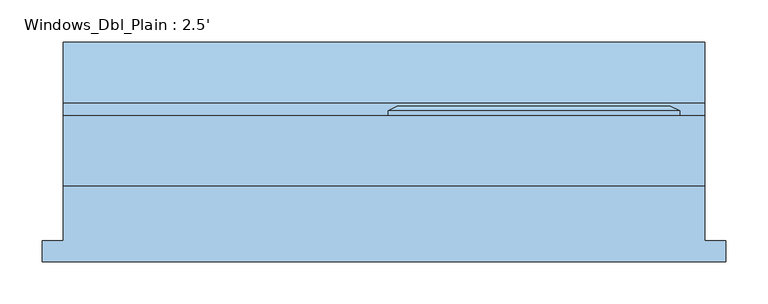
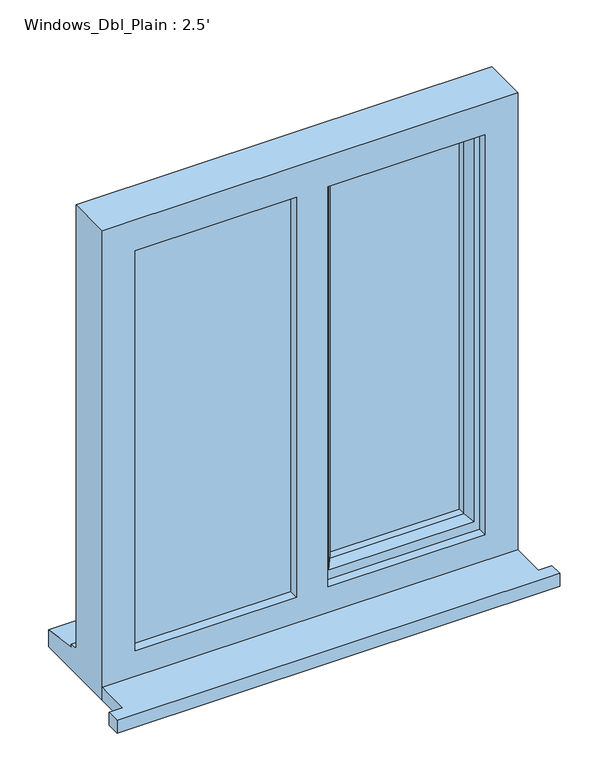
"""IFC4 building model written with IfcOpenShell, lengths in millimetres: window geometry, Windows_Dbl_Plain : 2.5'."""

from ifc_helpers import new_model, si_unit, frame, origin, place, context, project, spatial, polyline, outline, extrude, faceted_brep, source, transform, mapped, element, save


def windows_dbl_plain_2_5_52f1e8c5(model_context):
    return source(origin(), model_context, "Body", "SolidModel", [
        extrude(outline(polyline([(-691.0, -115.6034322), (-691.0, -90.6034322), (-666.0, -90.6034322), (-666.0, -25.4834322), (96.0, -25.4834322), (96.0, -90.6034322), (121.0, -90.6034322), (121.0, -115.6034322), (-691.0, -115.6034322)])), frame((0.0, 0.0, 1200.0), z_axis=(0.0, 0.0, 1.0), x_axis=(1.0, 0.0, 0.0)), (0.0, 0.0, 1.0), 25.0),
        faceted_brep([(-280.0, 57.5165678, 2080.0), (-280.0, 63.2900705, 2080.0), (-280.0, 63.2900705, 1253.0), (-280.0, 57.5165678, 1253.0), (-270.0, -7.4834322, 2070.0), (-270.0, 57.5165678, 2070.0), (-270.0, 57.5165678, 1263.0), (-270.0, -7.4834322, 1263.0), (-230.0, 7.0094677, 2030.0), (-240.1480377, -7.4834322, 2040.1480377), (-240.1480377, -7.4834322, 1292.8519623), (-230.0, 7.0094677, 1303.0), (-230.0, 21.5165678, 2030.0), (-230.0, 21.5165678, 1303.0), (-240.0, 45.5165678, 2040.0), (-240.0, 21.5165678, 2040.0), (-240.0, 21.5165678, 1293.0), (-240.0, 45.5165678, 1293.0), (-230.0, 63.2900705, 2030.0), (-230.0, 45.5165678, 2030.0), (-230.0, 45.5165678, 1303.0), (-230.0, 63.2900705, 1303.0), (-247.4457548, 69.0635732, 2047.4457548), (-247.4457548, 69.0635732, 1285.5542452), (-269.2153903, 69.0635732, 2069.2153903), (-269.2153903, 69.0635732, 1263.7846097), (66.0, 63.2900705, 1253.0), (66.0, 57.5165678, 1253.0), (56.0, 57.5165678, 1263.0), (56.0, -7.4834322, 1263.0), (26.1480377, -7.4834322, 1292.8519623), (16.0, 7.0094677, 1303.0), (16.0, 21.5165678, 1303.0), (26.0, 21.5165678, 1293.0), (26.0, 45.5165678, 1293.0), (16.0, 45.5165678, 1303.0), (16.0, 63.2900705, 1303.0), (33.4457548, 69.0635732, 1285.5542452), (55.2153903, 69.0635732, 1263.7846097), (66.0, 63.2900705, 2080.0), (66.0, 57.5165678, 2080.0), (56.0, 57.5165678, 2070.0), (56.0, -7.4834322, 2070.0), (26.1480377, -7.4834322, 2040.1480377), (16.0, 7.0094677, 2030.0), (16.0, 21.5165678, 2030.0), (26.0, 21.5165678, 2040.0), (26.0, 45.5165678, 2040.0), (16.0, 45.5165678, 2030.0), (16.0, 63.2900705, 2030.0), (33.4457548, 69.0635732, 2047.4457548), (55.2153903, 69.0635732, 2069.2153903)], [[[0, 1, 2, 3]], [[4, 5, 6, 7]], [[8, 9, 10, 11]], [[12, 8, 11, 13]], [[14, 15, 16, 17]], [[18, 19, 20, 21]], [[22, 18, 21, 23]], [[1, 24, 25, 2]], [[3, 2, 26, 27]], [[7, 6, 28, 29]], [[11, 10, 30, 31]], [[13, 11, 31, 32]], [[17, 16, 33, 34]], [[21, 20, 35, 36]], [[23, 21, 36, 37]], [[2, 25, 38, 26]], [[27, 26, 39, 40]], [[29, 28, 41, 42]], [[31, 30, 43, 44]], [[32, 31, 44, 45]], [[34, 33, 46, 47]], [[36, 35, 48, 49]], [[37, 36, 49, 50]], [[26, 38, 51, 39]], [[40, 39, 1, 0]], [[3, 27, 40, 0], [5, 41, 28, 6]], [[42, 41, 5, 4]], [[7, 29, 42, 4], [9, 43, 30, 10]], [[44, 43, 9, 8]], [[45, 44, 8, 12]], [[15, 46, 33, 16], [13, 32, 45, 12]], [[47, 46, 15, 14]], [[17, 34, 47, 14], [19, 48, 35, 20]], [[49, 48, 19, 18]], [[50, 49, 18, 22]], [[24, 51, 38, 25], [23, 37, 50, 22]], [[39, 51, 24, 1]]]),
        extrude(outline(polyline([(2050.0, -310.0), (2070.0, -310.0), (2070.0, -626.0), (1263.0, -626.0), (1263.0, -310.0), (1283.0, -310.0), (1283.0, -606.0), (2050.0, -606.0), (2050.0, -310.0)])), frame((0.0, 16.5165678, 0.0), z_axis=(0.0, 1.0, 0.0), x_axis=(0.0, 0.0, 1.0)), (0.0, 0.0, 1.0), 41.0),
        faceted_brep([(96.0, -25.4834322, 2110.0), (-666.0, -25.4834322, 2110.0), (-666.0, -25.4834322, 1200.0), (96.0, -25.4834322, 1200.0), (36.0, -25.4834322, 2050.0), (36.0, -25.4834322, 1275.0), (-252.0, -25.4834322, 1275.0), (-252.0, -25.4834322, 2050.0), (-310.0, -25.4834322, 2050.0), (-310.0, -25.4834322, 1275.0), (-606.0, -25.4834322, 1275.0), (-606.0, -25.4834322, 2050.0), (-666.0, 57.5165678, 2110.0), (-666.0, 57.5165678, 1251.0), (-666.0, 72.5165678, 1249.68767), (-666.0, 72.5165678, 1244.7449676), (-666.0, 145.0165678, 1233.8088847), (-666.0, 145.0165678, 1200.0), (96.0, 57.5165678, 2110.0), (96.0, 57.5165678, 1251.0), (-626.0, 57.5165678, 2070.0), (-626.0, 57.5165678, 1263.0), (-310.0, 57.5165678, 1263.0), (-310.0, 57.5165678, 2070.0), (-270.0, 57.5165678, 2070.0), (-270.0, 57.5165678, 1263.0), (56.0, 57.5165678, 1263.0), (56.0, 57.5165678, 2070.0), (-626.0, -7.4834322, 2070.0), (-626.0, -7.4834322, 1263.0), (-300.0, -7.4834322, 2070.0), (-300.0, -7.4834322, 1263.0), (-310.0, -7.4834322, 2050.0), (-606.0, -7.4834322, 2050.0), (-606.0, -7.4834322, 1275.0), (-310.0, -7.4834322, 1275.0), (-270.0, -7.4834322, 2070.0), (56.0, -7.4834322, 2070.0), (56.0, -7.4834322, 1263.0), (-270.0, -7.4834322, 1263.0), (36.0, -7.4834322, 2050.0), (-252.0, -7.4834322, 2050.0), (-252.0, -7.4834322, 1275.0), (36.0, -7.4834322, 1275.0), (-310.0, 16.5165678, 2070.0), (-300.0, 16.5165678, 2070.0), (96.0, 145.0165678, 1200.0), (96.0, 145.0165678, 1233.8088847), (96.0, 72.5165678, 1244.7449676), (96.0, 72.5165678, 1249.68767), (-300.0, 16.5165678, 1263.0), (-310.0, 16.5165678, 1263.0)], [[[0, 1, 2, 3], [4, 5, 6, 7], [8, 9, 10, 11]], [[2, 1, 12, 13, 14, 15, 16, 17]], [[13, 12, 18, 19], [20, 21, 22, 23], [24, 25, 26, 27]], [[21, 20, 28, 29]], [[28, 30, 31, 29], [32, 33, 34, 35]], [[36, 37, 38, 39], [40, 41, 42, 43]], [[33, 11, 10, 34]], [[1, 0, 18, 12]], [[28, 20, 23, 44, 45, 30]], [[27, 37, 36, 24]], [[11, 33, 32, 8]], [[40, 4, 7, 41]], [[19, 18, 0, 3, 46, 47, 48, 49]], [[27, 26, 38, 37]], [[4, 40, 43, 5]], [[45, 50, 31, 30]], [[50, 45, 44, 51]], [[51, 44, 23, 22]], [[25, 24, 36, 39]], [[41, 7, 6, 42]], [[8, 32, 35, 9]], [[46, 3, 2, 17]], [[47, 46, 17, 16]], [[48, 47, 16, 15]], [[49, 48, 15, 14]], [[19, 49, 14, 13]], [[22, 21, 29, 31, 50, 51]], [[26, 25, 39, 38]], [[6, 5, 43, 42]], [[35, 34, 10, 9]]]),
        extrude(outline(polyline([(-626.0, 16.5165678), (-300.0, 16.5165678), (-300.0, -7.4834322), (-626.0, -7.4834322), (-626.0, 16.5165678)])), frame((0.0, 0.0, 1263.0), z_axis=(0.0, 0.0, 1.0), x_axis=(1.0, 0.0, 0.0)), (0.0, 0.0, 1.0), 807.0),
        extrude(outline(polyline([(26.0, 21.5165678), (-240.0, 21.5165678), (-240.0, 45.5165678), (26.0, 45.5165678), (26.0, 21.5165678)])), frame((0.0, 0.0, 1293.0), z_axis=(0.0, 0.0, 1.0), x_axis=(1.0, 0.0, 0.0)), (0.0, 0.0, 1.0), 747.0),
    ])


if __name__ == "__main__":
    model = new_model("IFC4")
    model_context = context("Model", 3, world=origin())
    ifc_project = project(units=[si_unit("LENGTHUNIT", "METRE", prefix="MILLI")], contexts=[model_context])
    site = spatial("IfcSite", under=ifc_project)
    building = spatial("IfcBuilding", under=site)
    placement = place(None, origin())
    windows_dbl_plain_2_5_shape = windows_dbl_plain_2_5_52f1e8c5(model_context)
    element("IfcWindow", 1, ObjectType="Windows_Dbl_Plain : 2.5'", at=placement, inside=building, context=model_context, shape_type="MappedRepresentation", body=[
        mapped(windows_dbl_plain_2_5_shape, transform((0.0, 0.0, 0.0), x_axis=(1.0, 0.0, 0.0), y_axis=(0.0, 1.0, 0.0), z_axis=(0.0, 0.0, 1.0))),
    ])
    save(model, "model.ifc")

# Revit data of these elements
# Type "Windows_Dbl_Plain : 2.5'"
#   Type Mark = "57"
#   Operation = "DoublePanelVertical"
#   Construction Type Id = "GSP4R"
#   Manufacturer = "Revit"
#   Keynote = "L10"
#   Analytic Construction = "1/8 in Pilkington single glazing"
#   Wrap Layers (Ext) from Ext = 0.336286 ft
#   Wrap Layers (Int) from Ext = 0.582349 ft
#   Window Board Projection = 0.082021 ft
#   Window Board Extension = 0.082021 ft
#   Visual Light Transmittance = 0.9
#   Solar Heat Gain Coefficient = 0.78
#   Rough Width = 2.5 ft
#   Rough Height = 2.985564 ft
#   Height = 2.985564 ft
#   Width = 2.5 ft
#   Heat Transfer Coefficient (U) = 3.6886 W/(m²·K)
#   Glazing Thickness = 0.07874 ft
#   FrameOffset - External = 0.164042 ft
#   Frame Depth = 0.213255 ft
#   Default Head Height = 6.922572 ft
#   Cill Depth = 0.287073 ft
#   Cavity Closer Width = 0.164042 ft
#   Cavity Closer Offset from Ext = 0.336286 ft
#   Cavity Closer Depth = 0.278871 ft
#   Vis - Cavity Closers = yes
#   Define Thermal Properties by = 1
#   Material Trim = Window Frame
#   Material Glass = Glass
#   Material Frame = Window Frame
#   Wall Closure = (empty or 0)
# Element 1 (IfcWindow, "Windows_Dbl_Plain : 2.5'")
#   Materials on its faces: "Window Frame", "Glass"
# Materials
#   "Window Frame": colour RGB 249 249 249, transparency 0, Keynote = "L10", Cost = 0
#   "Glass": class "Glass", colour RGB 0 128 192, transparency 0.9, Description = "Soda Lime Glass", Cost = 0
